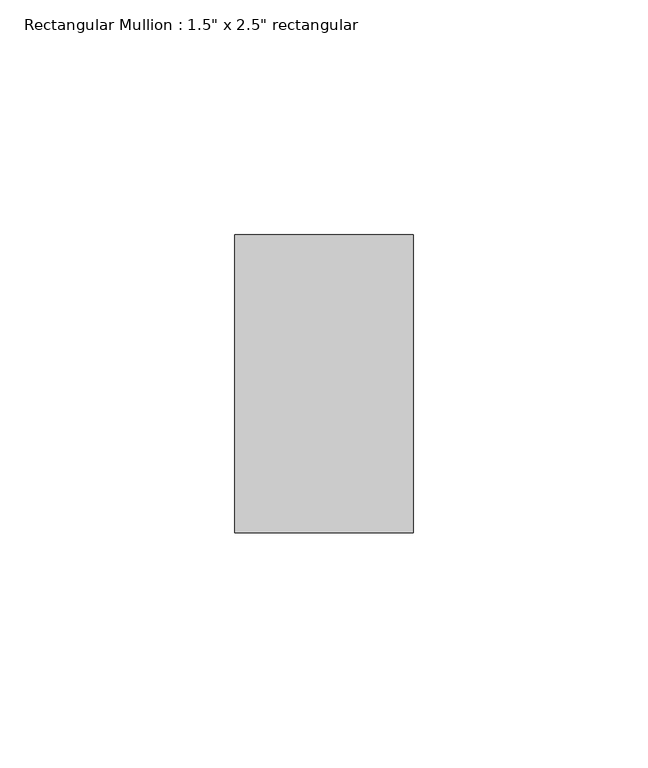
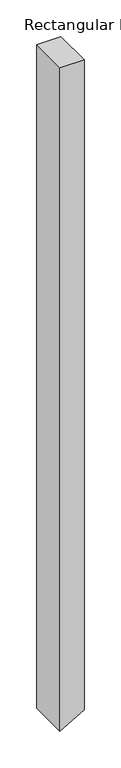
"""IFC4 building model written with IfcOpenShell, lengths in millimetres: member geometry."""

from ifc_helpers import new_model, si_unit, frame, origin, place, context, project, spatial, polyline, outline, extrude, source, transform, mapped, element, save


def member_eb314aa0(model_context):
    return source(origin(), model_context, "Body", "SweptSolid", [
        extrude(outline(polyline([(0.0, 19.05), (0.0, -19.05), (-1104.3176875, -19.05), (-1081.6731736, 19.05), (0.0, 19.05)])), frame((0.0, -31.75, 0.0), z_axis=(0.0, 1.0, 0.0), x_axis=(0.0, 0.0, 1.0)), (0.0, 0.0, 1.0), 63.5),
    ])


if __name__ == "__main__":
    model = new_model("IFC4")
    model_context = context("Model", 3, world=origin())
    ifc_project = project(units=[si_unit("LENGTHUNIT", "METRE", prefix="MILLI")], contexts=[model_context])
    site = spatial("IfcSite", under=ifc_project)
    building = spatial("IfcBuilding", under=site)
    placement = place(None, origin())
    member_shape = member_eb314aa0(model_context)
    element("IfcMember", 1, ObjectType="Rectangular Mullion : 1.5\" x 2.5\" rectangular", at=placement, inside=building, context=model_context, shape_type="MappedRepresentation", body=[
        mapped(member_shape, transform((0.0, 0.0, 0.0), x_axis=(1.0, 0.0, 0.0), y_axis=(0.0, 1.0, 0.0), z_axis=(0.0, 0.0, 1.0))),
    ])
    save(model, "model.ifc")

# Revit data of these elements
# Type "Rectangular Mullion : 1.5\" x 2.5\" rectangular"
#   built-in parameter 1007304 = 0.208333 (stored number, unit not read)
#   built-in parameter 1007301 = 0.0625 (stored number, unit not read)
#   built-in parameter 1007300 = 0.0625 (stored number, unit not read)
